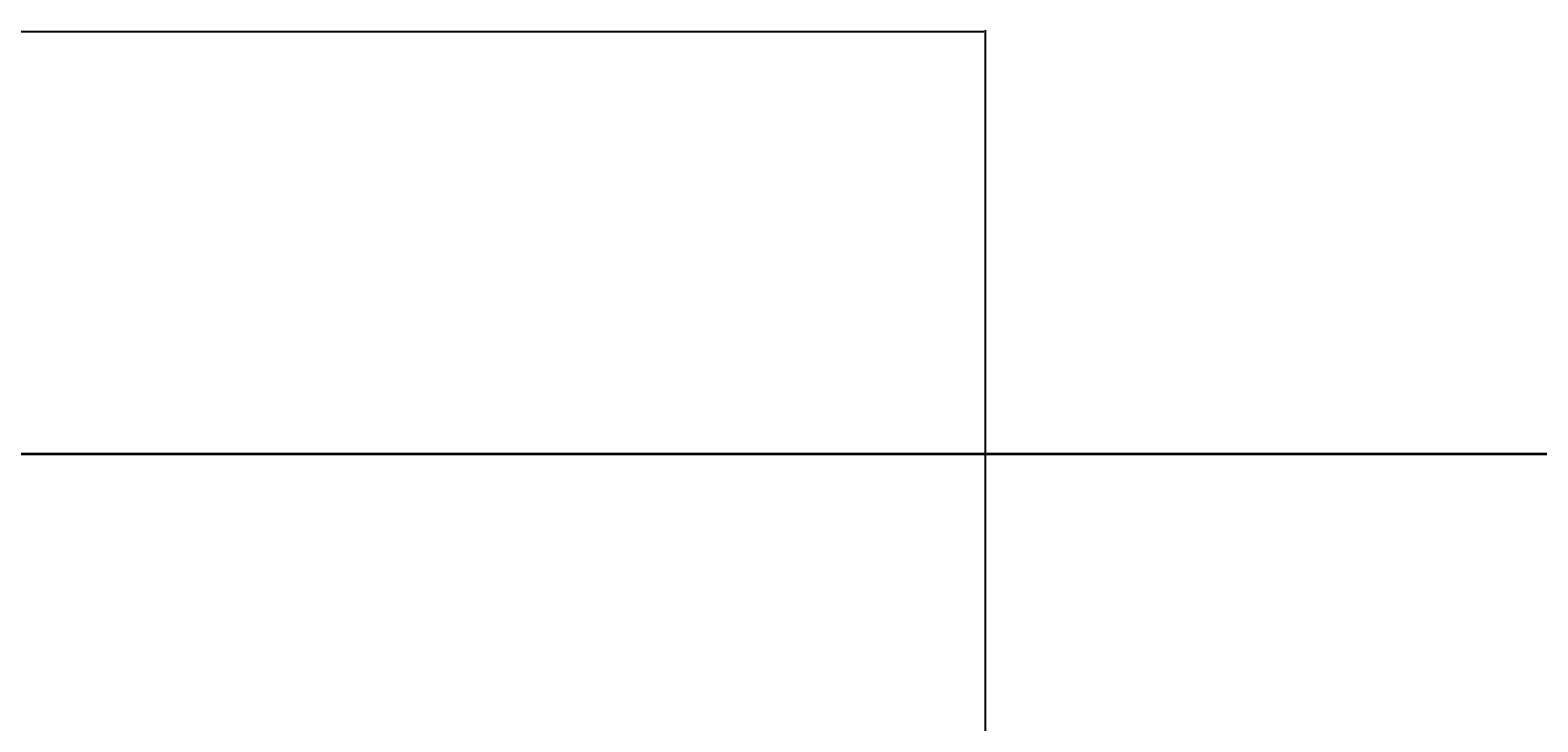
# Model space of a CAD drawing. Units: feet. Extents: x 2100 to 2836, y 2433 to 3396.
# Tile 11 of 12: x 2309 to 2468, y 3324 to 3396. Entities that reach past the tile are written whole.
import ezdxf

# ---------------------------------------------------------------- set-up
doc = ezdxf.new("R2010")
doc.units = ezdxf.units.FT
doc.layers.add('A-ANNO-DIMS', color=2, linetype='Continuous', lineweight=18)
doc.layers.add('A-ANNO-TTLB', color=7, linetype='Continuous', lineweight=35)
doc.styles.get("Standard").update_dxf_attribs({"font": 'arial.ttf'})
doc.dimstyles.get("Standard").update_dxf_attribs({"dimtxt": 0.18, "dimasz": 0.18, "dimexe": 0.18, "dimexo": 0.0625, "dimgap": 0.09, "dimtad": 0, "dimtih": 1, "dimtoh": 1, "dimdec": 4, "dimzin": 0, "dimdsep": 46, "dimtxsty": 'Standard', "dimcen": 0.09, "dimadec": 0, "dimazin": 0, "dimtfac": 1, "dimtdec": 4, "dimtofl": 0, "dimtmove": 0, "dimatfit": 3, "dimfxl": 1, "dimtolj": 1, "dimtzin": 0, "dimarcsym": 0})

# ---------------------------------------------------------------- blocks, each defined once
blk = doc.blocks.new('*D40')
at = {"layer": 'A-ANNO-DIMS', "color": 0, "lineweight": -2, "transparency": 16777216}
for p, q in [((2190.69, 3321.87), (2190.69, 3396.05)), ((2190.87, 3395.87), (2299.9, 3395.87)), ((2409.51, 3395.87), (2300.48, 3395.87)), ((2409.69, 3321.87), (2409.69, 3396.05))]:
    blk.add_line(p, q, dxfattribs=at)
at = {"layer": 'A-ANNO-DIMS', "color": 0, "transparency": 16777216}
for points in [[(2190.87, 3395.9), (2190.87, 3395.84), (2190.69, 3395.87)], [(2409.51, 3395.9), (2409.51, 3395.84), (2409.69, 3395.87)]]:
    blk.add_solid(points, dxfattribs=at)
at = {"layer": 'Defpoints', "color": 0, "transparency": 16777216}
for p in [(2409.69, 3395.87), (2190.69, 3321.8), (2409.69, 3321.8)]:
    blk.add_point(p, dxfattribs=at)
at = {"layer": 'A-ANNO-DIMS', "color": 0, "transparency": 16777216, "insert": (2300.19, 3395.87), "char_height": 0.18, "attachment_point": 5}
blk.add_mtext('\\A1;219', dxfattribs=at)

msp = doc.modelspace()

# ---------------------------------------------------------------- linework, layer by layer
at = {"layer": 'A-ANNO-TTLB'}
msp.add_lwpolyline([(2144.0848, 3351.6245), (2791.0561, 3351.6245), (2791.0561, 2477.4373), (2144.0848, 2477.4373)], close=True, dxfattribs=at)

# ---------------------------------------------------------------- dimensions: what is measured, and where the dimension line sits
at = {"layer": 'A-ANNO-DIMS'}
dim = msp.add_linear_dim(base=(2409.6857, 3395.8745), p1=(2190.6857, 3321.8031), p2=(2409.6857, 3321.8031), dimstyle='Standard', override={"dimdec": 0, "dimlfac": 1, "dimrnd": 0, "dimzin": 0, "dimdsep": 46, "dimlunit": 2}, dxfattribs=at)
dim.commit()
dim.dimension.update_dxf_attribs({"geometry": '*D40', "text_midpoint": (2300.1857, 3395.8745)})

doc.saveas('drawing.dxf')
